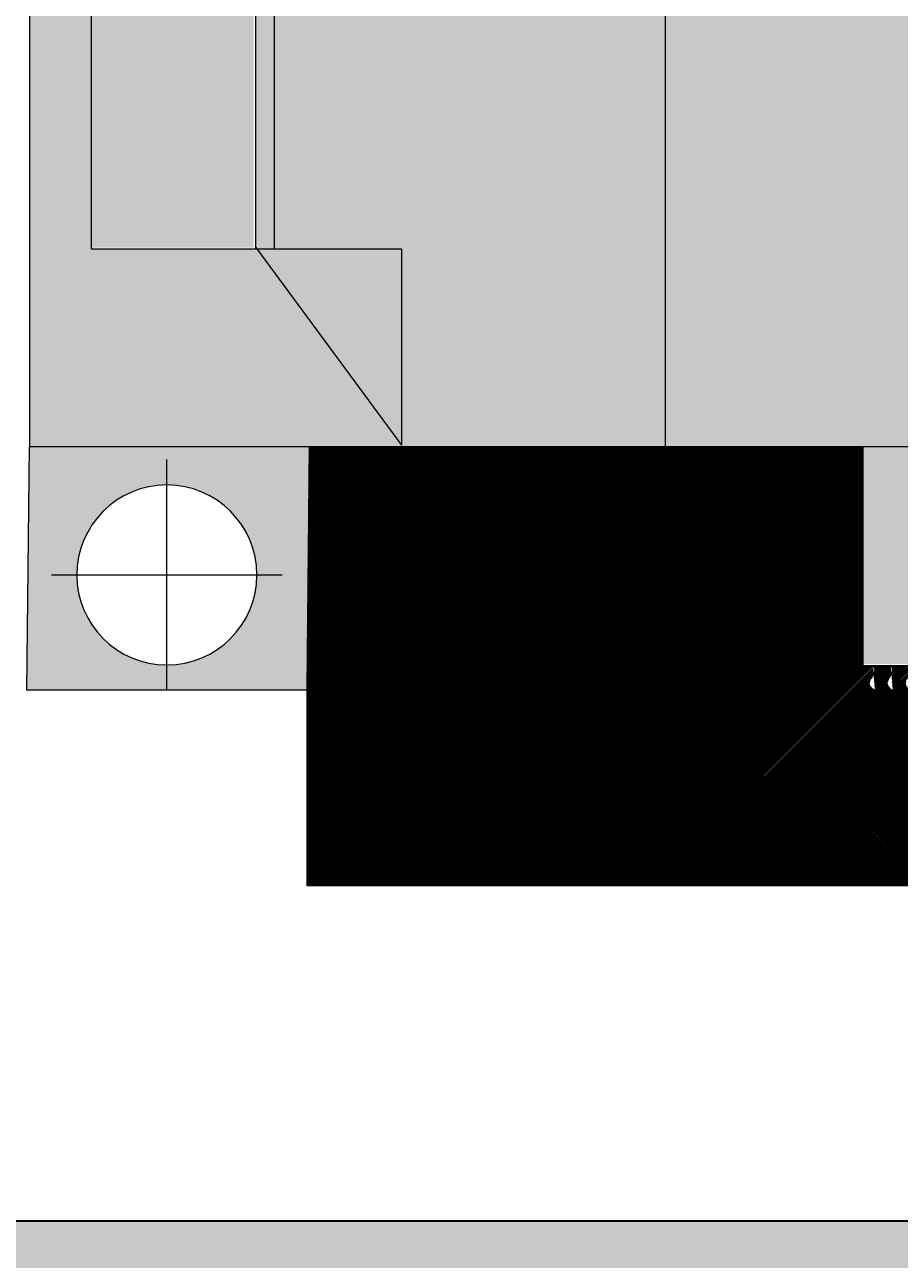
# Model space of a CAD drawing. Units: inches. Extents: x 192 to 1361, y -1362 to 367.
# Tile 4 of 23: x 293 to 396, y -761 to -616. Entities that reach past the tile are written whole.
import ezdxf

# ---------------------------------------------------------------- set-up
doc = ezdxf.new("R2010")
doc.units = ezdxf.units.IN
doc.header["$MEASUREMENT"] = 0
for name, color, linetype, lineweight in [('A-ANNO-DIMS', 2, 'Continuous', 18), ('A-FLOR', 8, 'Continuous', 18), ('A-WALL-PATT', 250, 'Continuous', 13), ('furniture', 32, 'Continuous', 18), ('walls', 7, 'Continuous', 35)]:
    doc.layers.add(name, color=color, linetype=linetype, lineweight=lineweight)
doc.layers.add('A-FLOR-PATT', color=254, linetype='Continuous', lineweight=13, true_color=0xfeeab9)
doc.layers.add('A-FURN-PATT', color=254, linetype='Continuous', lineweight=13, true_color=0xfeeab9)
doc.styles.get("Standard").update_dxf_attribs({"font": 'arial.ttf'})
doc.dimstyles.get("Standard").update_dxf_attribs({"dimtxt": 0.18, "dimasz": 0.18, "dimexe": 0.18, "dimexo": 0.0625, "dimgap": 0.09, "dimtad": 0, "dimtih": 1, "dimtoh": 1, "dimzin": 0, "dimdsep": 46, "dimlunit": 3, "dimtxsty": 'Standard', "dimcen": 0.09, "dimadec": 0, "dimazin": 0, "dimtfac": 1, "dimtofl": 0, "dimtmove": 0, "dimatfit": 3, "dimfxl": 1, "dimtolj": 1, "dimtzin": 0, "dimarcsym": 0})

# ---------------------------------------------------------------- blocks, each defined once
blk = doc.blocks.new('CARPET')
at = {"layer": 'furniture'}
for p, q in [((36, -55.124), (51.553, -55.124)), ((51.553, -55.124), (51.553, -98.109))]:
    blk.add_line(p, q, dxfattribs=at)
for points in [[(53.374, -55.995), (53.215, -55.797), (52.902, -55.407), (52.343, -55.797), (51.889, -56.079), (51.645, -55.906), (51.535, -55.827)], [(53.374, -57.263), (53.215, -57.065), (52.902, -56.675), (52.343, -57.065), (51.889, -57.347), (51.645, -57.174), (51.535, -57.095)]]:
    blk.add_open_spline(points, degree=3, knots=[0, 0, 0, 0, 0.653278, 1.290138, 1.740457, 2.114451, 2.114451, 2.114451, 2.114451], dxfattribs=at)
blk = doc.blocks.new('A$C58D270C6')
at = {"layer": 'furniture'}
for p, q in [((9.094, 124.131), (9.094, 108.869)), ((1.463, 116.5), (16.725, 116.5)), ((14.974, 94.844), (24.617, 107.922)), ((24.617, 94.932), (24.617, 107.922)), ((42.078, 108), (42.078, 36)), ((14.974, 94.932), (24.617, 94.932)), ((14.974, 94.844), (14.974, 36)), ((16.217, 94.932), (16.217, 36))]:
    blk.add_line(p, q, dxfattribs=at)
for points in [[(18.499, 108), (18.344, 124.131), (-0.156, 124.131), (0, 108)], [(0, 108), (77.905, 108), (77.905, 36), (0, 36)], [(4.094, 94.932), (14.974, 94.932), (14.974, 73.835), (4.094, 73.835)]]:
    blk.add_lwpolyline(points, close=True, dxfattribs=at)
blk.add_circle((9.094, 116.5), 5.955, dxfattribs=at)
at = {"layer": 'furniture', "xscale": 0.9312884925094044, "yscale": 0.9312884925094044, "zscale": 0.9312884925094044, "rotation": 90}
blk.add_blockref('CARPET', (3.79, 74.474), dxfattribs=at)
blk = doc.blocks.new('*D48')
at = {"layer": 'A-ANNO-DIMS', "color": 0, "lineweight": -2, "transparency": 16777216}
for p, q in [((325.63, 258.53), (192.16, 258.53)), ((192.34, 258.35), (192.34, -429.22)), ((192.34, -1117.14), (192.34, -429.58)), ((395.21, -1117.32), (192.16, -1117.32))]:
    blk.add_line(p, q, dxfattribs=at)
at = {"layer": 'A-ANNO-DIMS', "color": 0, "transparency": 16777216}
for points in [[(192.31, 258.35), (192.37, 258.35), (192.34, 258.53)], [(192.31, -1117.14), (192.37, -1117.14), (192.34, -1117.32)]]:
    blk.add_solid(points, dxfattribs=at)
at = {"layer": 'Defpoints', "color": 0, "transparency": 16777216}
for p in [(325.7, 258.53), (192.34, -1117.32), (395.28, -1117.32)]:
    blk.add_point(p, dxfattribs=at)
at = {"layer": 'A-ANNO-DIMS', "color": 0, "transparency": 16777216, "insert": (192.34, -429.4), "char_height": 0.18, "attachment_point": 5}
blk.add_mtext('\\A1;1375.9', dxfattribs=at)

msp = doc.modelspace()

# ---------------------------------------------------------------- hatches: boundary and pattern name
at = {"layer": 'A-FLOR-PATT'}
h = msp.add_hatch(dxfattribs=at)
h.set_pattern_fill('ANSI31', color=256)
edge = h.paths.add_edge_path()
edge.add_line((513.1511, -492.1899), (327.1032, -492.1899))
edge.add_line((327.1032, -492.1899), (327.1032, -508.439))
edge.add_line((327.1032, -508.439), (326.9465, -508.439))
edge.add_line((326.9465, -508.439), (326.6697, -537.1419))
edge.add_line((326.6697, -537.1419), (391.8439, -537.1419))
edge.add_line((391.8439, -537.1419), (391.8439, -520.2026))
edge.add_line((391.8439, -520.2026), (393.0084, -520.2026))
edge.add_spline(control_points=[(393.2858, -517.1545), (392.9584, -517.4172), (392.3119, -517.936), (392.9583, -518.8629), (393.4257, -519.6151), (393.1386, -520.0192), (393.0084, -520.2026)], knot_values=[0, 0, 0, 0, 0.65327829, 1.2901376, 1.74045698, 2.11445126, 2.11445126, 2.11445126, 2.11445126], degree=3, periodic=0)
edge.add_line((393.0084, -520.2026), (395.1098, -520.2026))
edge.add_spline(control_points=[(395.3872, -517.1545), (395.0598, -517.4172), (394.4133, -517.936), (395.0598, -518.8629), (395.5272, -519.6151), (395.2401, -520.0192), (395.1098, -520.2026)], knot_values=[0, 0, 0, 0, 0.65327829, 1.2901376, 1.74045698, 2.11445126, 2.11445126, 2.11445126, 2.11445126], degree=3, periodic=0)
edge.add_line((395.1098, -520.2026), (397.3144, -520.2026))
edge.add_spline(control_points=[(397.5918, -517.1545), (397.2644, -517.4172), (396.6179, -517.936), (397.2643, -518.8629), (397.7317, -519.6151), (397.4446, -520.0192), (397.3144, -520.2026)], knot_values=[0, 0, 0, 0, 0.65327829, 1.2901376, 1.74045698, 2.11445126, 2.11445126, 2.11445126, 2.11445126], degree=3, periodic=0)
edge.add_line((397.3144, -520.2026), (399.2806, -520.2026))
edge.add_spline(control_points=[(399.558, -517.1545), (399.2307, -517.4172), (398.5841, -517.936), (399.2306, -518.8629), (399.698, -519.6151), (399.4109, -520.0192), (399.2806, -520.2026)], knot_values=[0, 0, 0, 0, 0.65327829, 1.2901376, 1.74045698, 2.11445126, 2.11445126, 2.11445126, 2.11445126], degree=3, periodic=0)
edge.add_line((399.2806, -520.2026), (401.664, -520.2026))
edge.add_spline(control_points=[(401.9414, -517.1545), (401.614, -517.4172), (400.9675, -517.936), (401.6139, -518.8629), (402.0814, -519.6151), (401.7943, -520.0192), (401.664, -520.2026)], knot_values=[0, 0, 0, 0, 0.65327829, 1.2901376, 1.74045698, 2.11445126, 2.11445126, 2.11445126, 2.11445126], degree=3, periodic=0)
edge.add_line((401.664, -520.2026), (403.6961, -520.2026))
edge.add_spline(control_points=[(403.9735, -517.1545), (403.6461, -517.4172), (402.9996, -517.936), (403.6461, -518.8629), (404.1135, -519.6151), (403.8264, -520.0192), (403.6961, -520.2026)], knot_values=[0, 0, 0, 0, 0.65327829, 1.2901376, 1.74045698, 2.11445126, 2.11445126, 2.11445126, 2.11445126], degree=3, periodic=0)
edge.add_line((403.6961, -520.2026), (405.6624, -520.2026))
edge.add_spline(control_points=[(405.9398, -517.1545), (405.6124, -517.4172), (404.9659, -517.936), (405.6123, -518.8629), (406.0797, -519.6151), (405.7926, -520.0192), (405.6624, -520.2026)], knot_values=[0, 0, 0, 0, 0.65327829, 1.2901376, 1.74045698, 2.11445126, 2.11445126, 2.11445126, 2.11445126], degree=3, periodic=0)
edge.add_line((405.6624, -520.2026), (408.0457, -520.2026))
edge.add_spline(control_points=[(408.3231, -517.1545), (407.9958, -517.4172), (407.3493, -517.936), (407.9957, -518.8629), (408.4631, -519.6151), (408.176, -520.0192), (408.0457, -520.2026)], knot_values=[0, 0, 0, 0, 0.65327829, 1.2901376, 1.74045698, 2.11445126, 2.11445126, 2.11445126, 2.11445126], degree=3, periodic=0)
edge.add_line((408.0457, -520.2026), (410.8462, -520.2026))
edge.add_spline(control_points=[(411.1236, -517.1545), (410.7962, -517.4172), (410.1497, -517.936), (410.7961, -518.8629), (411.2635, -519.6151), (410.9764, -520.0192), (410.8462, -520.2026)], knot_values=[0, 0, 0, 0, 0.65327829, 1.2901376, 1.74045698, 2.11445126, 2.11445126, 2.11445126, 2.11445126], degree=3, periodic=0)
edge.add_line((410.8462, -520.2026), (413.2295, -520.2026))
edge.add_spline(control_points=[(413.5069, -517.1545), (413.1795, -517.4172), (412.533, -517.936), (413.1794, -518.8629), (413.6468, -519.6151), (413.3597, -520.0192), (413.2295, -520.2026)], knot_values=[0, 0, 0, 0, 0.65327829, 1.2901376, 1.74045698, 2.11445126, 2.11445126, 2.11445126, 2.11445126], degree=3, periodic=0)
edge.add_line((413.2295, -520.2026), (415.434, -520.2026))
edge.add_spline(control_points=[(415.7114, -517.1545), (415.3841, -517.4172), (414.7376, -517.936), (415.384, -518.8629), (415.8514, -519.6151), (415.5643, -520.0192), (415.434, -520.2026)], knot_values=[0, 0, 0, 0, 0.65327829, 1.2901376, 1.74045698, 2.11445126, 2.11445126, 2.11445126, 2.11445126], degree=3, periodic=0)
edge.add_line((415.434, -520.2026), (417.5321, -520.2026))
edge.add_spline(control_points=[(417.8095, -517.1545), (417.4821, -517.4172), (416.8356, -517.936), (417.482, -518.8629), (417.9494, -519.6151), (417.6623, -520.0192), (417.5321, -520.2026)], knot_values=[0, 0, 0, 0, 0.65327829, 1.2901376, 1.74045698, 2.11445126, 2.11445126, 2.11445126, 2.11445126], degree=3, periodic=0)
edge.add_line((417.5321, -520.2026), (419.7366, -520.2026))
edge.add_spline(control_points=[(420.014, -517.1545), (419.6867, -517.4172), (419.0401, -517.936), (419.6866, -518.8629), (420.154, -519.6151), (419.8669, -520.0192), (419.7366, -520.2026)], knot_values=[0, 0, 0, 0, 0.65327829, 1.2901376, 1.74045698, 2.11445126, 2.11445126, 2.11445126, 2.11445126], degree=3, periodic=0)
edge.add_line((419.7366, -520.2026), (421.7029, -520.2026))
edge.add_spline(control_points=[(421.9803, -517.1545), (421.6529, -517.4172), (421.0064, -517.936), (421.6528, -518.8629), (422.1202, -519.6151), (421.8331, -520.0192), (421.7029, -520.2026)], knot_values=[0, 0, 0, 0, 0.65327829, 1.2901376, 1.74045698, 2.11445126, 2.11445126, 2.11445126, 2.11445126], degree=3, periodic=0)
edge.add_line((421.7029, -520.2026), (424.0863, -520.2026))
edge.add_spline(control_points=[(424.3637, -517.1545), (424.0363, -517.4172), (423.3898, -517.936), (424.0362, -518.8629), (424.5036, -519.6151), (424.2165, -520.0192), (424.0863, -520.2026)], knot_values=[0, 0, 0, 0, 0.65327829, 1.2901376, 1.74045698, 2.11445126, 2.11445126, 2.11445126, 2.11445126], degree=3, periodic=0)
edge.add_line((424.0863, -520.2026), (426.1184, -520.2026))
edge.add_spline(control_points=[(426.3958, -517.1545), (426.0684, -517.4172), (425.4219, -517.936), (426.0683, -518.8629), (426.5357, -519.6151), (426.2486, -520.0192), (426.1184, -520.2026)], knot_values=[0, 0, 0, 0, 0.65327829, 1.2901376, 1.74045698, 2.11445126, 2.11445126, 2.11445126, 2.11445126], degree=3, periodic=0)
edge.add_line((426.1184, -520.2026), (428.0846, -520.2026))
edge.add_spline(control_points=[(428.362, -517.1545), (428.0346, -517.4172), (427.3881, -517.936), (428.0346, -518.8629), (428.502, -519.6151), (428.2149, -520.0192), (428.0846, -520.2026)], knot_values=[0, 0, 0, 0, 0.65327829, 1.2901376, 1.74045698, 2.11445126, 2.11445126, 2.11445126, 2.11445126], degree=3, periodic=0)
edge.add_line((428.0846, -520.2026), (430.468, -520.2026))
edge.add_spline(control_points=[(430.7454, -517.1545), (430.418, -517.4172), (429.7715, -517.936), (430.4179, -518.8629), (430.8853, -519.6151), (430.5983, -520.0192), (430.468, -520.2026)], knot_values=[0, 0, 0, 0, 0.65327829, 1.2901376, 1.74045698, 2.11445126, 2.11445126, 2.11445126, 2.11445126], degree=3, periodic=0)
edge.add_line((430.468, -520.2026), (433.2684, -520.2026))
edge.add_spline(control_points=[(433.5458, -517.1545), (433.2184, -517.4172), (432.5719, -517.936), (433.2184, -518.8629), (433.6858, -519.6151), (433.3987, -520.0192), (433.2684, -520.2026)], knot_values=[0, 0, 0, 0, 0.65327829, 1.2901376, 1.74045698, 2.11445126, 2.11445126, 2.11445126, 2.11445126], degree=3, periodic=0)
edge.add_line((433.2684, -520.2026), (435.6517, -520.2026))
edge.add_spline(control_points=[(435.9291, -517.1545), (435.6017, -517.4172), (434.9552, -517.936), (435.6017, -518.8629), (436.0691, -519.6151), (435.782, -520.0192), (435.6517, -520.2026)], knot_values=[0, 0, 0, 0, 0.65327829, 1.2901376, 1.74045698, 2.11445126, 2.11445126, 2.11445126, 2.11445126], degree=3, periodic=0)
edge.add_line((435.6517, -520.2026), (437.8563, -520.2026))
edge.add_spline(control_points=[(438.1337, -517.1545), (437.8063, -517.4172), (437.1598, -517.936), (437.8062, -518.8629), (438.2736, -519.6151), (437.9865, -520.0192), (437.8563, -520.2026)], knot_values=[0, 0, 0, 0, 0.65327829, 1.2901376, 1.74045698, 2.11445126, 2.11445126, 2.11445126, 2.11445126], degree=3, periodic=0)
edge.add_line((437.8563, -520.2026), (439.7189, -520.2026))
edge.add_spline(control_points=[(439.9963, -517.1545), (439.669, -517.4172), (439.0225, -517.936), (439.6689, -518.8629), (440.1363, -519.6151), (439.8492, -520.0192), (439.7189, -520.2026)], knot_values=[0, 0, 0, 0, 0.65327829, 1.2901376, 1.74045698, 2.11445126, 2.11445126, 2.11445126, 2.11445126], degree=3, periodic=0)
edge.add_line((439.7189, -520.2026), (441.9235, -520.2026))
edge.add_spline(control_points=[(442.2009, -517.1545), (441.8735, -517.4172), (441.227, -517.936), (441.8735, -518.8629), (442.3409, -519.6151), (442.0538, -520.0192), (441.9235, -520.2026)], knot_values=[0, 0, 0, 0, 0.65327829, 1.2901376, 1.74045698, 2.11445126, 2.11445126, 2.11445126, 2.11445126], degree=3, periodic=0)
edge.add_line((441.9235, -520.2026), (443.8898, -520.2026))
edge.add_spline(control_points=[(444.1672, -517.1545), (443.8398, -517.4172), (443.1933, -517.936), (443.8397, -518.8629), (444.3071, -519.6151), (444.02, -520.0192), (443.8898, -520.2026)], knot_values=[0, 0, 0, 0, 0.65327829, 1.2901376, 1.74045698, 2.11445126, 2.11445126, 2.11445126, 2.11445126], degree=3, periodic=0)
edge.add_line((443.8898, -520.2026), (446.2731, -520.2026))
edge.add_spline(control_points=[(446.5505, -517.1545), (446.2232, -517.4172), (445.5767, -517.936), (446.2231, -518.8629), (446.6905, -519.6151), (446.4034, -520.0192), (446.2731, -520.2026)], knot_values=[0, 0, 0, 0, 0.65327829, 1.2901376, 1.74045698, 2.11445126, 2.11445126, 2.11445126, 2.11445126], degree=3, periodic=0)
edge.add_line((446.2731, -520.2026), (448.3052, -520.2026))
edge.add_spline(control_points=[(448.5826, -517.1545), (448.2553, -517.4172), (447.6088, -517.936), (448.2552, -518.8629), (448.7226, -519.6151), (448.4355, -520.0192), (448.3052, -520.2026)], knot_values=[0, 0, 0, 0, 0.65327829, 1.2901376, 1.74045698, 2.11445126, 2.11445126, 2.11445126, 2.11445126], degree=3, periodic=0)
edge.add_line((448.3052, -520.2026), (450.2715, -520.2026))
edge.add_spline(control_points=[(450.5489, -517.1545), (450.2215, -517.4172), (449.575, -517.936), (450.2214, -518.8629), (450.6888, -519.6151), (450.4018, -520.0192), (450.2715, -520.2026)], knot_values=[0, 0, 0, 0, 0.65327829, 1.2901376, 1.74045698, 2.11445126, 2.11445126, 2.11445126, 2.11445126], degree=3, periodic=0)
edge.add_line((450.2715, -520.2026), (452.6549, -520.2026))
edge.add_spline(control_points=[(452.9323, -517.1545), (452.6049, -517.4172), (451.9584, -517.936), (452.6048, -518.8629), (453.0722, -519.6151), (452.7851, -520.0192), (452.6549, -520.2026)], knot_values=[0, 0, 0, 0, 0.65327829, 1.2901376, 1.74045698, 2.11445126, 2.11445126, 2.11445126, 2.11445126], degree=3, periodic=0)
edge.add_line((452.6549, -520.2026), (453.8151, -520.2026))
edge.add_spline(control_points=[(454.0925, -517.1545), (453.7499, -517.417), (453.0754, -517.9338), (453.769, -518.8576), (454.2314, -519.6154), (453.945, -520.0193), (453.8151, -520.2026)], knot_values=[0, 0, 0, 0, 0.6639037, 1.30740562, 1.757725, 2.13171928, 2.13171928, 2.13171928, 2.13171928], degree=3, periodic=0)
edge.add_line((453.8151, -520.2026), (455.3467, -520.2026))
edge.add_spline(control_points=[(455.6241, -517.1545), (455.2967, -517.4172), (454.6502, -517.936), (455.2967, -518.8629), (455.7641, -519.6151), (455.477, -520.0192), (455.3467, -520.2026)], knot_values=[0, 0, 0, 0, 0.65327829, 1.2901376, 1.74045698, 2.11445126, 2.11445126, 2.11445126, 2.11445126], degree=3, periodic=0)
edge.add_line((455.3467, -520.2026), (456.895, -520.2026))
edge.add_spline(control_points=[(456.895, -520.2026), (457.0253, -520.0192), (457.3124, -519.6151), (456.845, -518.8629), (456.1986, -517.936), (456.8451, -517.4172), (457.1724, -517.1545)], knot_values=[0, 0, 0, 0, 0.37399428, 0.82431366, 1.46117297, 2.11445126, 2.11445126, 2.11445126, 2.11445126], degree=3, periodic=0)
edge.add_spline(control_points=[(458.0074, -517.1545), (457.68, -517.4172), (457.0335, -517.936), (457.68, -518.8629), (458.1474, -519.6151), (457.8603, -520.0192), (457.73, -520.2026)], knot_values=[0, 0, 0, 0, 0.65327829, 1.2901376, 1.74045698, 2.11445126, 2.11445126, 2.11445126, 2.11445126], degree=3, periodic=0)
edge.add_line((457.73, -520.2026), (458.8613, -520.2026))
edge.add_spline(control_points=[(459.1387, -517.1545), (458.8113, -517.4172), (458.1648, -517.936), (458.8112, -518.8629), (459.2786, -519.6151), (458.9916, -520.0192), (458.8613, -520.2026)], knot_values=[0, 0, 0, 0, 0.65327829, 1.2901376, 1.74045698, 2.11445126, 2.11445126, 2.11445126, 2.11445126], degree=3, periodic=0)
edge.add_line((458.8613, -520.2026), (459.9346, -520.2026))
edge.add_spline(control_points=[(460.212, -517.1545), (459.8846, -517.4172), (459.2381, -517.936), (459.8845, -518.8629), (460.3519, -519.6151), (460.0648, -520.0192), (459.9346, -520.2026)], knot_values=[0, 0, 0, 0, 0.65327829, 1.2901376, 1.74045698, 2.11445126, 2.11445126, 2.11445126, 2.11445126], degree=3, periodic=0)
edge.add_line((459.9346, -520.2026), (461.2447, -520.2026))
edge.add_spline(control_points=[(461.5221, -517.1545), (461.1947, -517.4172), (460.5482, -517.936), (461.1946, -518.8629), (461.662, -519.6151), (461.3749, -520.0192), (461.2447, -520.2026)], knot_values=[0, 0, 0, 0, 0.65327829, 1.2901376, 1.74045698, 2.11445126, 2.11445126, 2.11445126, 2.11445126], degree=3, periodic=0)
edge.add_line((461.2447, -520.2026), (462.6002, -520.2026))
edge.add_spline(control_points=[(462.8776, -517.1545), (462.5502, -517.4172), (461.9037, -517.936), (462.5501, -518.8629), (463.0175, -519.6151), (462.7304, -520.0192), (462.6002, -520.2026)], knot_values=[0, 0, 0, 0, 0.65327829, 1.2901376, 1.74045698, 2.11445126, 2.11445126, 2.11445126, 2.11445126], degree=3, periodic=0)
edge.add_line((462.6002, -520.2026), (463.0739, -520.2026))
edge.add_line((463.0739, -520.2026), (463.0739, -691.0271))
edge.add_line((463.0739, -691.0271), (462.6214, -691.0271))
edge.add_spline(control_points=[(462.8776, -694.0453), (462.5502, -693.7826), (461.9037, -693.2638), (462.5501, -692.3369), (463.011, -691.5951), (462.7443, -691.2005), (462.6214, -691.0271)], knot_values=[0, 0, 0, 0, 0.65327829, 1.2901376, 1.74045698, 2.09412198, 2.09412198, 2.09412198, 2.09412198], degree=3, periodic=0)
edge.add_line((462.6214, -691.0271), (461.3416, -691.0271))
edge.add_spline(control_points=[(461.5978, -694.0453), (461.2704, -693.7826), (460.6239, -693.2638), (461.2703, -692.3369), (461.7312, -691.5951), (461.4644, -691.2005), (461.3416, -691.0271)], knot_values=[0, 0, 0, 0, 0.65327829, 1.2901376, 1.74045698, 2.09412198, 2.09412198, 2.09412198, 2.09412198], degree=3, periodic=0)
edge.add_line((461.3416, -691.0271), (460.0315, -691.0271))
edge.add_spline(control_points=[(460.2877, -694.0453), (459.9603, -693.7826), (459.3138, -693.2638), (459.9602, -692.3369), (460.4211, -691.5951), (460.1544, -691.2005), (460.0315, -691.0271)], knot_values=[0, 0, 0, 0, 0.65327829, 1.2901376, 1.74045698, 2.09412198, 2.09412198, 2.09412198, 2.09412198], degree=3, periodic=0)
edge.add_line((460.0315, -691.0271), (458.9582, -691.0271))
edge.add_spline(control_points=[(459.2144, -694.0453), (458.887, -693.7826), (458.2405, -693.2638), (458.8869, -692.3369), (459.3478, -691.5951), (459.0811, -691.2005), (458.9582, -691.0271)], knot_values=[0, 0, 0, 0, 0.65327829, 1.2901376, 1.74045698, 2.09412198, 2.09412198, 2.09412198, 2.09412198], degree=3, periodic=0)
edge.add_line((458.9582, -691.0271), (457.8269, -691.0271))
edge.add_spline(control_points=[(457.8269, -691.0271), (457.9464, -691.2008), (458.2187, -691.5966), (457.7545, -692.3366), (457.1096, -693.2638), (457.7558, -693.7826), (458.0831, -694.0453)], knot_values=[0, 0, 0, 0, 0.3521435, 0.80246288, 1.43932219, 2.09260048, 2.09260048, 2.09260048, 2.09260048], degree=3, periodic=0)
edge.add_spline(control_points=[(457.2481, -694.0453), (456.9209, -693.7826), (456.2746, -693.2638), (456.9195, -692.3366), (457.3837, -691.5966), (457.1114, -691.2008), (456.992, -691.0271)], knot_values=[0, 0, 0, 0, 0.65327829, 1.2901376, 1.74045698, 2.09260048, 2.09260048, 2.09260048, 2.09260048], degree=3, periodic=0)
edge.add_line((456.992, -691.0271), (455.4436, -691.0271))
edge.add_spline(control_points=[(455.6998, -694.0453), (455.3725, -693.7826), (454.7263, -693.2638), (455.3712, -692.3366), (455.8354, -691.5966), (455.5631, -691.2008), (455.4436, -691.0271)], knot_values=[0, 0, 0, 0, 0.65327829, 1.2901376, 1.74045698, 2.09260048, 2.09260048, 2.09260048, 2.09260048], degree=3, periodic=0)
edge.add_line((455.4436, -691.0271), (453.8363, -691.0271))
edge.add_spline(control_points=[(454.0925, -694.0453), (453.7602, -693.7827), (453.1046, -693.2646), (453.7653, -692.3383), (454.2277, -691.5965), (453.9557, -691.2008), (453.8363, -691.0271)], knot_values=[0, 0, 0, 0, 0.65679228, 1.29582582, 1.7461452, 2.0982924, 2.0982924, 2.0982924, 2.0982924], degree=3, periodic=0)
edge.add_line((453.8363, -691.0271), (452.6761, -691.0271))
edge.add_spline(control_points=[(452.9323, -694.0453), (452.605, -693.7826), (451.9587, -693.2638), (452.6037, -692.3366), (453.0678, -691.5966), (452.7956, -691.2008), (452.6761, -691.0271)], knot_values=[0, 0, 0, 0, 0.65327829, 1.2901376, 1.74045698, 2.09260048, 2.09260048, 2.09260048, 2.09260048], degree=3, periodic=0)
edge.add_line((452.6761, -691.0271), (450.2927, -691.0271))
edge.add_spline(control_points=[(450.5489, -694.0453), (450.2216, -693.7826), (449.5753, -693.2638), (450.2203, -692.3366), (450.6845, -691.5966), (450.4122, -691.2008), (450.2927, -691.0271)], knot_values=[0, 0, 0, 0, 0.65327829, 1.2901376, 1.74045698, 2.09260048, 2.09260048, 2.09260048, 2.09260048], degree=3, periodic=0)
edge.add_line((450.2927, -691.0271), (448.3265, -691.0271))
edge.add_spline(control_points=[(448.5826, -694.0453), (448.2553, -693.7826), (447.6088, -693.2638), (448.2552, -692.3369), (448.7161, -691.5951), (448.4493, -691.2005), (448.3265, -691.0271)], knot_values=[0, 0, 0, 0, 0.65327829, 1.2901376, 1.74045698, 2.09412198, 2.09412198, 2.09412198, 2.09412198], degree=3, periodic=0)
edge.add_line((448.3265, -691.0271), (446.2944, -691.0271))
edge.add_spline(control_points=[(446.5505, -694.0453), (446.2232, -693.7826), (445.5767, -693.2638), (446.2231, -692.3369), (446.684, -691.5951), (446.4172, -691.2005), (446.2944, -691.0271)], knot_values=[0, 0, 0, 0, 0.65327829, 1.2901376, 1.74045698, 2.09412198, 2.09412198, 2.09412198, 2.09412198], degree=3, periodic=0)
edge.add_line((446.2944, -691.0271), (443.911, -691.0271))
edge.add_spline(control_points=[(444.1672, -694.0453), (443.8398, -693.7826), (443.1933, -693.2638), (443.8397, -692.3369), (444.3006, -691.5951), (444.0338, -691.2005), (443.911, -691.0271)], knot_values=[0, 0, 0, 0, 0.65327829, 1.2901376, 1.74045698, 2.09412198, 2.09412198, 2.09412198, 2.09412198], degree=3, periodic=0)
edge.add_line((443.911, -691.0271), (441.9447, -691.0271))
edge.add_spline(control_points=[(442.2009, -694.0453), (441.8735, -693.7826), (441.227, -693.2638), (441.8735, -692.3369), (442.3344, -691.5951), (442.0676, -691.2005), (441.9447, -691.0271)], knot_values=[0, 0, 0, 0, 0.65327829, 1.2901376, 1.74045698, 2.09412198, 2.09412198, 2.09412198, 2.09412198], degree=3, periodic=0)
edge.add_line((441.9447, -691.0271), (439.7402, -691.0271))
edge.add_spline(control_points=[(439.9963, -694.0453), (439.669, -693.7826), (439.0225, -693.2638), (439.6689, -692.3369), (440.1298, -691.5951), (439.863, -691.2005), (439.7402, -691.0271)], knot_values=[0, 0, 0, 0, 0.65327829, 1.2901376, 1.74045698, 2.09412198, 2.09412198, 2.09412198, 2.09412198], degree=3, periodic=0)
edge.add_line((439.7402, -691.0271), (437.8775, -691.0271))
edge.add_spline(control_points=[(438.1337, -694.0453), (437.8063, -693.7826), (437.1598, -693.2638), (437.8062, -692.3369), (438.2671, -691.5951), (438.0004, -691.2005), (437.8775, -691.0271)], knot_values=[0, 0, 0, 0, 0.65327829, 1.2901376, 1.74045698, 2.09412198, 2.09412198, 2.09412198, 2.09412198], degree=3, periodic=0)
edge.add_line((437.8775, -691.0271), (435.6729, -691.0271))
edge.add_spline(control_points=[(435.9291, -694.0453), (435.6017, -693.7826), (434.9552, -693.2638), (435.6017, -692.3369), (436.0626, -691.5951), (435.7958, -691.2005), (435.6729, -691.0271)], knot_values=[0, 0, 0, 0, 0.65327829, 1.2901376, 1.74045698, 2.09412198, 2.09412198, 2.09412198, 2.09412198], degree=3, periodic=0)
edge.add_line((435.6729, -691.0271), (433.2896, -691.0271))
edge.add_spline(control_points=[(433.5458, -694.0453), (433.2184, -693.7826), (432.5719, -693.2638), (433.2184, -692.3369), (433.6793, -691.5951), (433.4125, -691.2005), (433.2896, -691.0271)], knot_values=[0, 0, 0, 0, 0.65327829, 1.2901376, 1.74045698, 2.09412198, 2.09412198, 2.09412198, 2.09412198], degree=3, periodic=0)
edge.add_line((433.2896, -691.0271), (430.4892, -691.0271))
edge.add_spline(control_points=[(430.7454, -694.0453), (430.418, -693.7826), (429.7715, -693.2638), (430.4179, -692.3369), (430.8788, -691.5951), (430.6121, -691.2005), (430.4892, -691.0271)], knot_values=[0, 0, 0, 0, 0.65327829, 1.2901376, 1.74045698, 2.09412198, 2.09412198, 2.09412198, 2.09412198], degree=3, periodic=0)
edge.add_line((430.4892, -691.0271), (428.1058, -691.0271))
edge.add_spline(control_points=[(428.362, -694.0453), (428.0346, -693.7826), (427.3881, -693.2638), (428.0346, -692.3369), (428.4955, -691.5951), (428.2287, -691.2005), (428.1058, -691.0271)], knot_values=[0, 0, 0, 0, 0.65327829, 1.2901376, 1.74045698, 2.09412198, 2.09412198, 2.09412198, 2.09412198], degree=3, periodic=0)
edge.add_line((428.1058, -691.0271), (426.1396, -691.0271))
edge.add_spline(control_points=[(426.3958, -694.0453), (426.0684, -693.7826), (425.4219, -693.2638), (426.0683, -692.3369), (426.5292, -691.5951), (426.2624, -691.2005), (426.1396, -691.0271)], knot_values=[0, 0, 0, 0, 0.65327829, 1.2901376, 1.74045698, 2.09412198, 2.09412198, 2.09412198, 2.09412198], degree=3, periodic=0)
edge.add_line((426.1396, -691.0271), (424.1075, -691.0271))
edge.add_spline(control_points=[(424.3637, -694.0453), (424.0363, -693.7826), (423.3898, -693.2638), (424.0362, -692.3369), (424.4971, -691.5951), (424.2303, -691.2005), (424.1075, -691.0271)], knot_values=[0, 0, 0, 0, 0.65327829, 1.2901376, 1.74045698, 2.09412198, 2.09412198, 2.09412198, 2.09412198], degree=3, periodic=0)
edge.add_line((424.1075, -691.0271), (421.7241, -691.0271))
edge.add_spline(control_points=[(421.9803, -694.0453), (421.6529, -693.7826), (421.0064, -693.2638), (421.6528, -692.3369), (422.1137, -691.5951), (421.847, -691.2005), (421.7241, -691.0271)], knot_values=[0, 0, 0, 0, 0.65327829, 1.2901376, 1.74045698, 2.09412198, 2.09412198, 2.09412198, 2.09412198], degree=3, periodic=0)
edge.add_line((421.7241, -691.0271), (419.7579, -691.0271))
edge.add_spline(control_points=[(420.014, -694.0453), (419.6867, -693.7826), (419.0401, -693.2638), (419.6866, -692.3369), (420.1475, -691.5951), (419.8807, -691.2005), (419.7579, -691.0271)], knot_values=[0, 0, 0, 0, 0.65327829, 1.2901376, 1.74045698, 2.09412198, 2.09412198, 2.09412198, 2.09412198], degree=3, periodic=0)
edge.add_line((419.7579, -691.0271), (417.5533, -691.0271))
edge.add_spline(control_points=[(417.8095, -694.0453), (417.4821, -693.7826), (416.8356, -693.2638), (417.482, -692.3369), (417.9429, -691.5951), (417.6761, -691.2005), (417.5533, -691.0271)], knot_values=[0, 0, 0, 0, 0.65327829, 1.2901376, 1.74045698, 2.09412198, 2.09412198, 2.09412198, 2.09412198], degree=3, periodic=0)
edge.add_line((417.5533, -691.0271), (415.4553, -691.0271))
edge.add_spline(control_points=[(415.7114, -694.0453), (415.3841, -693.7826), (414.7376, -693.2638), (415.384, -692.3369), (415.8449, -691.5951), (415.5781, -691.2005), (415.4553, -691.0271)], knot_values=[0, 0, 0, 0, 0.65327829, 1.2901376, 1.74045698, 2.09412198, 2.09412198, 2.09412198, 2.09412198], degree=3, periodic=0)
edge.add_line((415.4553, -691.0271), (413.2507, -691.0271))
edge.add_spline(control_points=[(413.5069, -694.0453), (413.1795, -693.7826), (412.533, -693.2638), (413.1794, -692.3369), (413.6403, -691.5951), (413.3736, -691.2005), (413.2507, -691.0271)], knot_values=[0, 0, 0, 0, 0.65327829, 1.2901376, 1.74045698, 2.09412198, 2.09412198, 2.09412198, 2.09412198], degree=3, periodic=0)
edge.add_line((413.2507, -691.0271), (410.8674, -691.0271))
edge.add_spline(control_points=[(411.1236, -694.0453), (410.7962, -693.7826), (410.1497, -693.2638), (410.7961, -692.3369), (411.257, -691.5951), (410.9903, -691.2005), (410.8674, -691.0271)], knot_values=[0, 0, 0, 0, 0.65327829, 1.2901376, 1.74045698, 2.09412198, 2.09412198, 2.09412198, 2.09412198], degree=3, periodic=0)
edge.add_line((410.8674, -691.0271), (408.067, -691.0271))
edge.add_spline(control_points=[(408.3231, -694.0453), (407.9958, -693.7826), (407.3493, -693.2638), (407.9957, -692.3369), (408.4566, -691.5951), (408.1898, -691.2005), (408.067, -691.0271)], knot_values=[0, 0, 0, 0, 0.65327829, 1.2901376, 1.74045698, 2.09412198, 2.09412198, 2.09412198, 2.09412198], degree=3, periodic=0)
edge.add_line((408.067, -691.0271), (405.6836, -691.0271))
edge.add_spline(control_points=[(405.9398, -694.0453), (405.6124, -693.7826), (404.9659, -693.2638), (405.6123, -692.3369), (406.0732, -691.5951), (405.8064, -691.2005), (405.6836, -691.0271)], knot_values=[0, 0, 0, 0, 0.65327829, 1.2901376, 1.74045698, 2.09412198, 2.09412198, 2.09412198, 2.09412198], degree=3, periodic=0)
edge.add_line((405.6836, -691.0271), (403.7173, -691.0271))
edge.add_spline(control_points=[(403.9735, -694.0453), (403.6461, -693.7826), (402.9996, -693.2638), (403.6461, -692.3369), (404.107, -691.5951), (403.8402, -691.2005), (403.7173, -691.0271)], knot_values=[0, 0, 0, 0, 0.65327829, 1.2901376, 1.74045698, 2.09412198, 2.09412198, 2.09412198, 2.09412198], degree=3, periodic=0)
edge.add_line((403.7173, -691.0271), (401.6852, -691.0271))
edge.add_spline(control_points=[(401.9414, -694.0453), (401.614, -693.7826), (400.9675, -693.2638), (401.6139, -692.3369), (402.0749, -691.5951), (401.8081, -691.2005), (401.6852, -691.0271)], knot_values=[0, 0, 0, 0, 0.65327829, 1.2901376, 1.74045698, 2.09412198, 2.09412198, 2.09412198, 2.09412198], degree=3, periodic=0)
edge.add_line((401.6852, -691.0271), (399.3019, -691.0271))
edge.add_spline(control_points=[(399.558, -694.0453), (399.2307, -693.7826), (398.5841, -693.2638), (399.2306, -692.3369), (399.6915, -691.5951), (399.4247, -691.2005), (399.3019, -691.0271)], knot_values=[0, 0, 0, 0, 0.65327829, 1.2901376, 1.74045698, 2.09412198, 2.09412198, 2.09412198, 2.09412198], degree=3, periodic=0)
edge.add_line((399.3019, -691.0271), (397.3356, -691.0271))
edge.add_spline(control_points=[(397.5918, -694.0453), (397.2644, -693.7826), (396.6179, -693.2638), (397.2643, -692.3369), (397.7252, -691.5951), (397.4585, -691.2005), (397.3356, -691.0271)], knot_values=[0, 0, 0, 0, 0.65327829, 1.2901376, 1.74045698, 2.09412198, 2.09412198, 2.09412198, 2.09412198], degree=3, periodic=0)
edge.add_line((397.3356, -691.0271), (395.131, -691.0271))
edge.add_spline(control_points=[(395.3872, -694.0453), (395.0598, -693.7826), (394.4133, -693.2638), (395.0598, -692.3369), (395.5207, -691.5951), (395.2539, -691.2005), (395.131, -691.0271)], knot_values=[0, 0, 0, 0, 0.65327829, 1.2901376, 1.74045698, 2.09412198, 2.09412198, 2.09412198, 2.09412198], degree=3, periodic=0)
edge.add_line((395.131, -691.0271), (393.0296, -691.0271))
edge.add_spline(control_points=[(393.2858, -694.0453), (392.9584, -693.7826), (392.3119, -693.2638), (392.9583, -692.3369), (393.4192, -691.5951), (393.1524, -691.2005), (393.0296, -691.0271)], knot_values=[0, 0, 0, 0, 0.65327829, 1.2901376, 1.74045698, 2.09412198, 2.09412198, 2.09412198, 2.09412198], degree=3, periodic=0)
edge.add_line((393.0296, -691.0271), (391.8439, -691.0271))
edge.add_line((391.8439, -691.0271), (391.8439, -665.2551))
edge.add_line((391.8439, -665.2551), (326.6697, -665.2551))
edge.add_line((326.6697, -665.2551), (326.3929, -693.958))
edge.add_line((326.3929, -693.958), (326.3929, -716.9381))
edge.add_line((326.3929, -716.9381), (513.1511, -716.9381))
edge.add_line((513.1511, -716.9381), (513.1511, -492.1899))
h.paths.add_polyline_path([(353.9763, -588.1534), (487.3258, -588.1534), (487.3258, -561.3965), (353.9763, -561.3965)], flags=25)
at = {"layer": 'A-FURN-PATT'}
h = msp.add_hatch(color=256, dxfattribs=at)
h.dxf.hatch_style = 1
h.paths.add_polyline_path([(320.5124, -642.0022), (301.0388, -642.0022), (301.0388, -604.4633), (320.3977, -604.4633), (320.3977, -589.1472), (301.0388, -589.1472), (301.0388, -551.6082), (320.3977, -551.6082), (320.3977, -537.1419), (293.7534, -537.1419), (293.7534, -665.2551), (337.5553, -665.2551), (337.5553, -665.117)])
h.paths.add_polyline_path([(320.5305, -680.3795, -0.41421356), (309.9348, -690.9753), (309.9348, -693.958), (326.3929, -693.958), (326.6697, -665.2551), (293.7534, -665.2551), (293.4767, -693.958), (309.9348, -693.958), (309.9348, -690.9753, -0.41421356), (299.3391, -680.3795, -1)])
h.paths.add_polyline_path([(320.8073, -523.5634, -0.41421356), (310.2116, -534.1591), (310.2116, -537.1419), (326.6697, -537.1419), (326.9465, -508.439), (294.0302, -508.439), (293.7534, -537.1419), (310.2116, -537.1419), (310.2116, -534.1591, -0.41421356), (299.6159, -523.5634, -1)])
h = msp.add_hatch(color=256, dxfattribs=at)
h.dxf.hatch_style = 1
h.paths.add_polyline_path([(320.1552, -604.3144), (300.7962, -604.3144), (300.7962, -641.8533), (320.1552, -641.8533)])
h.paths.add_polyline_path([(320.1552, -551.4593), (300.7962, -551.4593), (300.7962, -588.9983), (320.1552, -588.9983)])
h.paths.add_polyline_path([(462.8313, -520.0537), (391.6014, -520.0537), (391.6014, -536.993), (432.1311, -536.993), (432.1311, -665.1062), (391.6014, -665.1062), (391.6014, -690.8782), (462.8313, -690.8782)])
h = msp.add_hatch(color=256, dxfattribs=at)
h.dxf.hatch_style = 1
h.paths.add_polyline_path([(337.5553, -642.0022), (320.5124, -642.0022), (337.5553, -665.117)])
h.paths.add_polyline_path([(322.6088, -537.1419), (320.3977, -537.1419), (320.3977, -641.8467), (320.5124, -642.0022), (322.6088, -642.0022)])
h = msp.add_hatch(color=256, dxfattribs=at)
h.dxf.hatch_style = 1
h.paths.add_polyline_path([(432.3737, -537.1419), (368.625, -537.1419), (368.625, -665.2551), (432.3737, -665.2551)])
h.paths.add_polyline_path([(368.625, -537.1419), (322.6088, -537.1419), (322.6088, -642.0022), (337.5553, -642.0022), (337.5553, -665.2551), (368.625, -665.2551)])
at = {"layer": 'A-WALL-PATT'}
h = msp.add_hatch(color=256, dxfattribs=at)
h.dxf.hatch_style = 1
h.paths.add_polyline_path([(309.5452, 191.102), (300.5452, 191.102), (300.5452, -126.898), (309.5452, -126.898), (309.5452, -117.898)])
h.paths.add_polyline_path([(420.798, 191.102), (337.3229, 191.102), (337.3229, 182.102), (420.798, 182.102)])
h.paths.add_polyline_path([(518.5452, 182.102), (625.4022, 182.102), (625.4022, 191.102), (509.5452, 191.102), (509.5452, 114.3262), (518.5452, 114.3262)])
h.paths.add_polyline_path([(842.5452, 191.102), (763.4438, 191.102), (763.4438, 182.102), (833.5452, 182.102), (833.5452, 161.1615), (836.8088, 161.1615), (842.5452, 161.1615)])
h.paths.add_polyline_path([(842.5452, -16.5675), (833.5452, -16.5675), (833.5452, -60.4996), (784.8041, -60.4996), (784.8041, -354.6796), (793.8041, -354.6796), (793.8041, -69.4996), (1094.1252, -69.4996), (1094.1252, -60.4996), (842.5452, -60.4996)])
h.paths.add_polyline_path([(518.5452, 36.602), (509.5452, 36.602), (509.5452, -117.898), (420.2204, -117.898), (420.2204, -126.898), (518.5452, -126.898)])
h.paths.add_polyline_path([(474.8041, -377.0384), (465.8041, -377.0384), (465.8041, -381.5384), (465.8041, -450.898), (537.5717, -450.898), (537.5717, -441.898), (474.8041, -441.898)])
h.paths.add_polyline_path([(1162.8041, -380.6763), (1204.3001, -380.6763), (1204.3001, -375.6763), (1195.1471, -375.6763), (1153.8041, -375.6763), (1153.8041, -448.4996), (856.5691, -448.4996), (856.5691, -457.4996), (1162.8041, -457.4996)])
h.paths.add_polyline_path([(1162.8041, -525.128), (1153.8041, -525.128), (1153.8041, -597.4996), (1162.8041, -597.4996)], flags=17)
h.paths.add_polyline_path([(1162.8041, -60.4996), (1153.8041, -60.4996), (1153.8041, -69.4996), (1153.8041, -177.4733), (1205.8889, -177.4733), (1205.8889, -172.4733), (1162.8041, -172.4733)])
h.paths.add_polyline_path([(980.5799, -525.686), (971.5799, -525.686), (971.5799, -597.4996), (980.5799, -597.4996)], flags=17)
h.paths.add_polyline_path([(856.5691, -448.4996), (798.7542, -448.4996), (784.8041, -448.4996), (784.8041, -457.4996), (847.5691, -457.4996), (847.5691, -597.4996), (784.8041, -597.4996), (784.8041, -606.4996), (1273.5658, -606.4996), (1273.5658, -597.4996), (856.5691, -597.4996)])
h.paths.add_polyline_path([(1273.5658, -773.892), (1099.8366, -773.892), (1099.8366, -851.9362), (1108.8366, -851.9362), (1108.8366, -782.892), (1273.5658, -782.892)])
h.paths.add_polyline_path([(1108.8366, -982.9214), (1099.8366, -982.9214), (1099.8366, -1067.6246), (1037.7563, -1067.6246), (1037.7563, -1076.6246), (1108.8366, -1076.6246)])
h.paths.add_polyline_path([(835.078, -1067.6246), (758.8458, -1067.6246), (758.8458, -940.2324), (749.8458, -940.2324), (749.8458, -963.172), (749.8458, -970.4644), (749.8458, -1076.6246), (835.078, -1076.6246)])
h.paths.add_polyline_path([(450.307, -1066.9838), (441.307, -1066.9838), (441.307, -1076.6246), (450.307, -1076.6246)])
h.paths.add_polyline_path([(492.8925, -756.4415), (274.8925, -756.4415), (274.8925, -765.4415), (492.8925, -765.4415)])
h.paths.add_polyline_path([(283.8925, -835.2244), (274.8925, -835.2244), (274.8925, -914.4415), (492.8925, -914.4415), (492.8925, -839.9415), (483.8925, -839.9415), (483.8925, -905.4415), (283.8925, -905.4415)])
h.paths.add_polyline_path([(283.8925, -441.898), (283.8925, -375.4296), (281.6021, -375.4296), (281.6021, -399.4121), (274.8925, -399.4121), (274.8925, -441.898), (274.8925, -684.5089), (283.8925, -684.5089)])

# ---------------------------------------------------------------- linework, layer by layer
at = {"layer": 'A-FLOR'}
for p, q in [((326.3929, -693.958), (326.3929, -716.9381)), ((326.3929, -716.9381), (513.1511, -716.9381))]:
    msp.add_line(p, q, dxfattribs=at)
at = {"layer": 'walls'}
msp.add_line((492.8925, -756.4415), (274.8925, -756.4415), dxfattribs=at)

# ---------------------------------------------------------------- block references
at = {"layer": 'furniture', "xscale": -1.779350280135438, "yscale": 1.779350280135438, "zscale": 1.779350280135438, "rotation": 180}
msp.add_blockref('A$C58D270C6', (293.7534, -473.0852), dxfattribs=at)

# ---------------------------------------------------------------- dimensions: what is measured, and where the dimension line sits
at = {"layer": 'A-ANNO-DIMS'}
dim = msp.add_linear_dim(base=(192.3425, -1117.3227), p1=(325.6957, 258.5286), p2=(395.2768, -1117.3227), angle=90, dimstyle='Standard', override={"dimdec": 1, "dimlfac": 1, "dimrnd": 0, "dimzin": 0, "dimdsep": 46, "dimlunit": 2}, dxfattribs=at)
dim.commit()
dim.dimension.update_dxf_attribs({"geometry": '*D48', "text_midpoint": (192.3425, -429.3971)})

doc.saveas('drawing.dxf')
